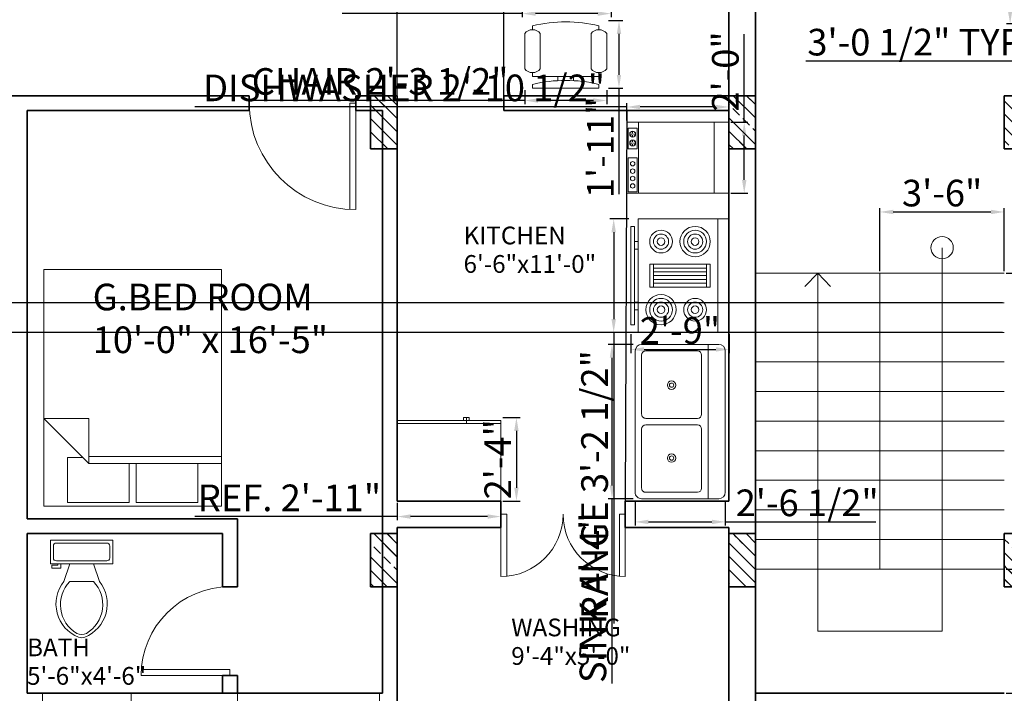
# Model space of a CAD drawing. Units: inches. Extents: x 2081 to 4786, y 1256 to 3802.
# Tile 3 of 7: x 2352 to 2685, y 1442 to 1670. Entities that reach past the tile are written whole.
import ezdxf

# ---------------------------------------------------------------- set-up
doc = ezdxf.new("R2010")
doc.units = ezdxf.units.IN
for name, color, linetype, lineweight in [('A-ANNO-DIMS', 18, 'Continuous', 18), ('A-AREA-IDEN', 18, 'Continuous', 18), ('A-COLS', 1, 'Continuous', 35), ('A-DOOR', 5, 'Continuous', 18), ('A-EQPM', 11, 'Continuous', 18), ('A-FLOR-CASE', 7, 'Continuous', 25), ('A-FLOR-FIXT', 18, 'Continuous', 18), ('A-FLOR-STRS', 7, 'Continuous', 18), ('A-FURN', 5, 'Continuous', 18), ('A-GLAZ', 11, 'Continuous', 18), ('A-WALL', 7, 'Continuous', 35)]:
    doc.layers.add(name, color=color, linetype=linetype, lineweight=lineweight)
doc.styles.get("Standard").update_dxf_attribs({"font": 'arial.ttf'})
doc.dimstyles.new('ISO-25', dxfattribs={"dimtxt": 9, "dimasz": 4.5, "dimexe": 1.25, "dimexo": 0.625, "dimtad": 1, "dimdec": 0, "dimlunit": 3, "dimtxsty": 'Standard', "dimcen": 2.5, "dimadec": 0, "dimazin": 0, "dimtfac": 1, "dimtdec": 0, "dimtmove": 0, "dimatfit": 3, "dimfxl": 1, "dimarcsym": 0})
pattern_1 = [(135, (1916.44, -3174.735), (-13.47038, -13.47038), []), (135, (1916.44, -3170.245), (-13.47038, -13.47038), []), (135, (1916.44, -3165.755), (-13.47038, -13.47038), []), (135, (1916.44, -3161.265), (-13.47038, -13.47038), [])]

# ---------------------------------------------------------------- blocks, each defined once
blk = doc.blocks.new('Bed - Queen')
for p, q in [((0, -80.00003), (0, 0)), ((0, 0), (59.99999, 0)), ((59.99999, 0), (59.99999, -80.00003)), ((7.99999, -1.2), (28.79998, -1.2)), ((7.99999, -14.4), (7.99999, -1.2)), ((28.79998, -1.2), (28.79998, -14.4)), ((31.19999, -1.2), (51.99999, -1.2)), ((31.19999, -14.4), (31.19999, -1.2)), ((51.99999, -1.2), (51.99999, -16.4)), ((0, -14.4), (44.8, -14.4)), ((59.99999, -29.6), (44.8, -14.4)), ((44.8, -14.4), (44.8, -29.6)), ((51.99999, -16.4), (46.79936, -16.4)), ((44.8, -16.8), (0, -16.8)), ((44.8, -29.6), (59.99999, -29.6)), ((59.99999, -80.00003), (0, -80.00003))]:
    blk.add_line(p, q)
blk = doc.blocks.new('Chair - Desk')
for p, q in [((-8.5, 0), (-8.5, -1)), ((-8.5, 0), (8.5, 0)), ((8.5, 0), (8.5, -1)), ((-2, -3), (-2, -1.9355)), ((2, -1.9576), (2, -3)), ((-10.5, -5), (-10.5, -14)), ((-8.5, -3), (-8.5, -4)), ((-8.5, -3), (8.5, -3)), ((-6.5, -14), (-6.5, -5)), ((6.5, -5), (6.5, -14)), ((8.5, -3), (8.5, -4)), ((10.5, -14), (10.5, -5)), ((-8.5, -15), (-8.5, -16)), ((8.5, -15), (8.5, -16))]:
    blk.add_line(p, q)
for centre, radius, start, end in [((0, 34.625), 36.625, 256.5803, 283.4197), ((-8.5, -6.5), 2.5, 36.8699, 143.1301), ((8.5, -6.5), 2.5, 36.8699, 143.1301), ((-8.5, -12.5), 2.5, 216.8699, 323.1301), ((8.5, -12.5), 2.5, 216.8699, 323.1301), ((0, 19.625), 36.625, 256.5803, 283.4197)]:
    blk.add_arc(centre, radius, start, end)
blk = doc.blocks.new('Range-Oven - 30 in top')
for p, q in [((0, -3), (30, -3)), ((12, -6), (18, -6)), ((13, -20), (13, -6)), ((14, -6), (14, -20)), ((15, -20), (15, -6)), ((16, -6), (16, -20)), ((17, -20), (17, -6)), ((18, -20), (12, -20)), ((6, -24), (6, -25)), ((8, -25), (8, -24)), ((22, -25), (22, -24)), ((24, -24), (24, -25))]:
    blk.add_line(p, q)
for points in [[(0, -24), (0, 0), (30, 0), (30, -24)], [(12, -21), (12, -5), (18, -5), (18, -21)], [(2, -26), (2, -25), (28, -25), (28, -26)]]:
    blk.add_lwpolyline(points, close=True)
for centre, radius in [((6, -9), 4), ((6, -9), 3), ((6, -9), 2), ((24, -9), 3), ((24, -9), 2), ((6, -9), 1), ((24, -9), 1), ((6, -18), 3), ((24, -18), 4), ((24, -18), 3), ((6, -18), 2), ((6, -18), 1), ((24, -18), 2), ((24, -18), 1)]:
    blk.add_circle(centre, radius)
blk = doc.blocks.new('Refrigerator-2 door - 36 in top')
for p, q in [((0, -26.999999), (36, -26.999999)), ((12, -26.999999), (12, -28.999999)), ((11, -27.999999), (11, -28.999999)), ((11, -28.999999), (13, -28.999999)), ((13, -28.999999), (13, -27.999999))]:
    blk.add_line(p, q)
blk.add_lwpolyline([(0, -27.999999), (0, 0), (36, 0), (36, -27.999999)], close=True)
blk = doc.blocks.new('Dishwasher')
for p, q in [((17, 32.75), (17, 33.5)), ((20, 32.75), (20, 33.5)), ((24, 30.5), (0, 30.5)), ((16, 32.5), (16.75, 32.5)), ((16.5, 32), (16.2942, 31.7942)), ((16.3156, 33.1843), (16.5, 33)), ((17, 32.25), (17, 31.5)), ((18, 32.5), (17.25, 32.5)), ((17.5, 33), (17.6938, 33.1938)), ((17.7061, 31.7939), (17.5, 32)), ((19, 32.5), (19.75, 32.5)), ((19.5, 32), (19.2942, 31.7942)), ((19.3156, 33.1843), (19.5, 33)), ((20, 32.25), (20, 31.5)), ((21, 32.5), (20.25, 32.5)), ((20.5, 33), (20.6938, 33.1938)), ((20.7061, 31.7939), (20.5, 32)), ((0, 5), (24, 5))]:
    blk.add_line(p, q)
for points in [[(0, 0), (0, 34.5), (24, 34.5), (24, 0)], [(0.5, 31), (0.5, 34), (12, 34), (12, 31)], [(15, 31), (15, 34), (22, 34), (22, 31)]]:
    blk.add_lwpolyline(points, close=True)
for centre, radius in [((17, 32.5), 1), ((20, 32.5), 1), ((2.5, 32.5), 0.75), ((5, 32.5), 0.75), ((7.5, 32.5), 0.75), ((10, 32.5), 0.75)]:
    blk.add_circle(centre, radius)
blk = doc.blocks.new('Sink-double - 36 in top')
for p, q in [((-18, -4), (18, -4)), ((-0.75, -18.5), (-0.75, -6.5)), ((0.75, -6.5), (0.75, -18.5))]:
    blk.add_line(p, q)
for points in [[(-16.5, 0), (16.5, 0)], [(-18, -19.5), (-18, -1.5)], [(18, -1.5), (18, -19.5)], [(-16.5, -18.5), (-16.5, -6.5)], [(-15.5, -5.5), (-1.75, -5.5)], [(1.75, -5.5), (15.5, -5.5)], [(16.5, -6.5), (16.5, -18.5)], [(-1.75, -19.5), (-15.5, -19.5)], [(15.5, -19.5), (1.75, -19.5)], [(16.5, -21), (-16.5, -21)]]:
    blk.add_lwpolyline(points)
for centre, radius in [((-8.5, -12.5), 1), ((-8.5, -12.5), 0.5), ((8.5, -12.5), 1), ((8.5, -12.5), 0.5)]:
    blk.add_circle(centre, radius)
for centre, radius, start, end in [((-16.5, -1.5), 1.5, 90, 180), ((16.5, -1.5), 1.5, 0, 90), ((-15.5, -6.5), 1, 90, 180), ((-1.75, -6.5), 1, 0, 90), ((1.75, -6.5), 1, 90, 180), ((15.5, -6.5), 1, 0, 90), ((-16.5, -19.5), 1.5, 180, 270), ((-15.5, -18.5), 1, 180, 270), ((-1.75, -18.5), 1, 270, 0), ((1.75, -18.5), 1, 180, 270), ((15.5, -18.5), 1, 270, 0), ((16.5, -19.5), 1.5, 270, 0)]:
    blk.add_arc(centre, radius, start, end)
blk = doc.blocks.new('Toilet - top')
for p, q in [((9.5, -6), (9.5, -2)), ((-10, -8.5), (-8, -8.5)), ((-10, -9.5), (-10, -8.5)), ((-7, -9.5), (-10, -9.5)), ((-8, -8.5), (-8, -8)), ((-7, -8), (-7, -9.5)), ((-4, -8), (-6, -14)), ((4, -8), (6, -14)), ((4, -14), (-4, -14))]:
    blk.add_line(p, q)
blk.add_lwpolyline([(10.5, -8), (10.5, 0), (-10.5, 0), (-10.5, -8)], close=True)
for points in [[(-9.5, -2), (-9.5, -6)], [(8.5, -1), (-8.5, -1)], [(-8.5, -7), (8.5, -7)]]:
    blk.add_lwpolyline(points)
for centre, radius, start, end in [((-8.62, -1.88), 0.884, 81.8699, 188.1301), ((8.62, -1.88), 0.884, 351.8699, 98.1301), ((-8.62, -6.12), 0.884, 171.8699, 278.1301), ((8.62, -6.12), 0.884, 261.8699, 8.1301), ((3.52, -21.58), 12.17, 141.4691, 247.9714), ((4.2, -21.82), 11.33, 136.3677, 238.9468), ((-3.52, -21.58), 12.17, 292.0284, 38.5307), ((-4.2, -21.82), 11.33, 301.053, 43.6321), ((0, -27.88), 4, 245.7318, 294.2682), ((0, -29), 4, 254.8605, 285.1395)]:
    blk.add_arc(centre, radius, start, end)
blk = doc.blocks.new('*D16')
at = {"layer": 'A-ANNO-DIMS', "color": 0, "lineweight": -2, "transparency": 16777216}
for p, q in [((2642.98, 1584.8), (2642.98, 1606.11)), ((2684.98, 1584.8), (2684.98, 1606.11)), ((2647.48, 1604.86), (2680.48, 1604.86))]:
    blk.add_line(p, q, dxfattribs=at)
at = {"layer": 'A-ANNO-DIMS', "color": 0, "transparency": 16777216}
for points in [[(2647.48, 1605.61), (2647.48, 1604.11), (2642.98, 1604.86)], [(2680.48, 1605.61), (2680.48, 1604.11), (2684.98, 1604.86)]]:
    blk.add_solid(points, dxfattribs=at)
at = {"layer": 'Defpoints', "color": 0, "transparency": 16777216}
for p in [(2684.98, 1604.86), (2642.98, 1584.17), (2684.98, 1584.17)]:
    blk.add_point(p, dxfattribs=at)
at = {"layer": 'A-ANNO-DIMS', "color": 0, "transparency": 16777216, "insert": (2663.98, 1610.08), "char_height": 9, "attachment_point": 5}
blk.add_mtext('3\'-6"', dxfattribs=at)
blk = doc.blocks.new('DOOR-PAIR-42IN')
for p, q in [((0, 42), (21, 42)), ((0, 40), (21, 40)), ((21, 42), (21, 40)), ((0, 2), (21, 2)), ((21, 0), (21, 2)), ((0, 0), (21, 0))]:
    blk.add_line(p, q)
for centre, start, end in [((21, 42), 180, 270), ((21, 0), 90, 180)]:
    blk.add_arc(centre, 21, start, end)
blk = doc.blocks.new('DOOR-SINGLE-36IN')
for p, q in [((34, 36), (34, 0)), ((36, 36), (36, 0)), ((36, 0), (34, 0))]:
    blk.add_line(p, q)
blk.add_arc((36, 0), 36, 90, 180)
blk = doc.blocks.new('DOOR-SINGLE-30IN')
for p, q in [((0, 30), (30, 30)), ((30, 30), (30, 28)), ((0, 28), (30, 28))]:
    blk.add_line(p, q)
blk.add_arc((30, 30), 30, 180, 270)
blk = doc.blocks.new('WINDOW-48IN')
for p, q in [((0, 0), (0, 9)), ((0, 9), (4, 9)), ((4, 9), (48, 9)), ((48, 0), (48, 9)), ((48, 6), (0, 6)), ((48, 4.5), (0, 4.5)), ((48, 3), (0, 3)), ((48, 0), (0, 0))]:
    blk.add_line(p, q)
blk = doc.blocks.new('WINDOW-30IN')
for p, q in [((0, 0), (0, 30)), ((0, 30), (9, 30)), ((3, 0), (3, 30)), ((4.5, 0), (4.5, 30)), ((6, 0), (6, 30)), ((9, 30), (9, 0)), ((9, 0), (0, 0))]:
    blk.add_line(p, q)
blk = doc.blocks.new('COLUMN-9X18IN')
h = blk.add_hatch()
h.set_pattern_fill('ANSI34', color=256, angle=90)
h.set_pattern_definition(pattern_1)
h.paths.add_polyline_path([(9, 18), (0, 18), (0, 0), (9, 0)])
h = blk.add_hatch()
h.set_pattern_fill('ANSI34', color=256, angle=90)
h.set_pattern_definition(pattern_1)
h.paths.add_polyline_path([(9, 18), (0, 18), (0, 0), (9, 0)])
h = blk.add_hatch()
h.set_pattern_fill('ANSI34', color=256, angle=90)
h.set_pattern_definition(pattern_1)
h.paths.add_polyline_path([(9, 18), (0, 18), (0, 0), (9, 0)])
h = blk.add_hatch()
h.set_pattern_fill('ANSI33', color=256, angle=90)
h.set_pattern_definition([(135, (1916.44, -3174.7355), (-4.490128, -4.490128), []), (135, (1916.44, -3170.2454), (-4.490128, -4.490128), [3.175, -1.5875])])
h.paths.add_polyline_path([(0, 0), (9, 0), (9, 18), (0, 18)])
for p, q in [((0, 0), (0, 18)), ((0, 18), (9, 18)), ((9, 18), (9, 0)), ((9, 0), (0, 0))]:
    blk.add_line(p, q)
blk = doc.blocks.new('*D53')
at = {"layer": 'A-ANNO-DIMS', "color": 0, "lineweight": -2, "transparency": 16777216}
for p, q in [((2523.02, 1646.06), (2523.02, 1641.28)), ((2550.71, 1646.06), (2550.71, 1641.28)), ((2523.02, 1642.53), (2429.87, 1642.53)), ((2546.21, 1642.53), (2527.52, 1642.53))]:
    blk.add_line(p, q, dxfattribs=at)
at = {"layer": 'A-ANNO-DIMS', "color": 0, "transparency": 16777216}
for points in [[(2527.52, 1643.28), (2527.52, 1641.78), (2523.02, 1642.53)], [(2546.21, 1643.28), (2546.21, 1641.78), (2550.71, 1642.53)]]:
    blk.add_solid(points, dxfattribs=at)
at = {"layer": 'Defpoints', "color": 0, "transparency": 16777216}
for p in [(2523.02, 1646.68), (2550.71, 1646.68), (2523.02, 1642.53)]:
    blk.add_point(p, dxfattribs=at)
at = {"layer": 'A-ANNO-DIMS', "color": 0, "transparency": 16777216, "insert": (2474.2, 1647.81), "char_height": 9, "attachment_point": 5}
blk.add_mtext('CHAIR 2\'-3 1/2"', dxfattribs=at)
blk = doc.blocks.new('*D54')
at = {"layer": 'A-ANNO-DIMS', "color": 0, "lineweight": -2, "transparency": 16777216}
for p, q in [((2551.33, 1669.53), (2556.11, 1669.53)), ((2554.86, 1665.03), (2554.86, 1651.18)), ((2551.33, 1646.68), (2556.11, 1646.68)), ((2554.86, 1646.68), (2554.86, 1610.86))]:
    blk.add_line(p, q, dxfattribs=at)
at = {"layer": 'A-ANNO-DIMS', "color": 0, "transparency": 16777216}
for points in [[(2554.11, 1665.03), (2555.61, 1665.03), (2554.86, 1669.53)], [(2554.11, 1651.18), (2555.61, 1651.18), (2554.86, 1646.68)]]:
    blk.add_solid(points, dxfattribs=at)
at = {"layer": 'Defpoints', "color": 0, "transparency": 16777216}
for p in [(2550.71, 1669.53), (2550.71, 1646.68), (2554.86, 1646.68)]:
    blk.add_point(p, dxfattribs=at)
at = {"layer": 'A-ANNO-DIMS', "color": 0, "transparency": 16777216, "insert": (2549.72, 1626.52), "char_height": 9, "attachment_point": 5, "rotation": 90}
blk.add_mtext('1\'-11"', dxfattribs=at)
blk = doc.blocks.new('*D55')
at = {"layer": 'A-ANNO-DIMS', "color": 0, "lineweight": -2, "transparency": 16777216}
for p, q in [((2686.95, 1752.41), (2686.95, 1850.7)), ((2698.93, 1752.41), (2685.7, 1752.41)), ((2686.95, 1672.91), (2686.95, 1747.91)), ((2698.93, 1668.41), (2685.7, 1668.41))]:
    blk.add_line(p, q, dxfattribs=at)
at = {"layer": 'A-ANNO-DIMS', "color": 0, "transparency": 16777216}
for points in [[(2686.2, 1747.91), (2687.7, 1747.91), (2686.95, 1752.41)], [(2686.2, 1672.91), (2687.7, 1672.91), (2686.95, 1668.41)]]:
    blk.add_solid(points, dxfattribs=at)
at = {"layer": 'Defpoints', "color": 0, "transparency": 16777216}
for p in [(2686.95, 1752.41), (2699.55, 1752.41), (2699.55, 1668.41)]:
    blk.add_point(p, dxfattribs=at)
at = {"layer": 'A-ANNO-DIMS', "color": 0, "transparency": 16777216, "insert": (2681.67, 1803.8), "char_height": 9, "attachment_point": 5, "rotation": 90}
blk.add_mtext('SOFA 7\'-0" TYP.', dxfattribs=at)
blk = doc.blocks.new('*D56')
at = {"layer": 'A-ANNO-DIMS', "color": 0, "lineweight": -2, "transparency": 16777216}
for p, q in [((2699.55, 1667.78), (2699.55, 1654.56)), ((2736.22, 1667.78), (2736.22, 1654.56)), ((2699.55, 1655.81), (2617.98, 1655.81)), ((2731.72, 1655.81), (2704.05, 1655.81))]:
    blk.add_line(p, q, dxfattribs=at)
at = {"layer": 'A-ANNO-DIMS', "color": 0, "transparency": 16777216}
for points in [[(2704.05, 1656.56), (2704.05, 1655.06), (2699.55, 1655.81)], [(2731.72, 1656.56), (2731.72, 1655.06), (2736.22, 1655.81)]]:
    blk.add_solid(points, dxfattribs=at)
at = {"layer": 'Defpoints', "color": 0, "transparency": 16777216}
for p in [(2699.55, 1668.41), (2736.22, 1668.41), (2699.55, 1655.81)]:
    blk.add_point(p, dxfattribs=at)
at = {"layer": 'A-ANNO-DIMS', "color": 0, "transparency": 16777216, "insert": (2656.52, 1661.09), "char_height": 9, "attachment_point": 5}
blk.add_mtext('3\'-0 1/2" TYP.', dxfattribs=at)
blk = doc.blocks.new('*D58')
at = {"layer": 'A-ANNO-DIMS', "color": 0, "lineweight": -2, "transparency": 16777216}
for p, q in [((2522.19, 1680.27), (2522.19, 1670.65)), ((2552.19, 1680.27), (2552.19, 1670.65)), ((2522.19, 1671.9), (2461.43, 1671.9)), ((2547.69, 1671.9), (2526.69, 1671.9))]:
    blk.add_line(p, q, dxfattribs=at)
at = {"layer": 'A-ANNO-DIMS', "color": 0, "transparency": 16777216}
for points in [[(2526.69, 1672.65), (2526.69, 1671.15), (2522.19, 1671.9)], [(2547.69, 1672.65), (2547.69, 1671.15), (2552.19, 1671.9)]]:
    blk.add_solid(points, dxfattribs=at)
at = {"layer": 'Defpoints', "color": 0, "transparency": 16777216}
for p in [(2522.19, 1680.9), (2552.19, 1680.9), (2522.19, 1671.9)]:
    blk.add_point(p, dxfattribs=at)
at = {"layer": 'A-ANNO-DIMS', "color": 0, "transparency": 16777216, "insert": (2489.56, 1677.12), "char_height": 9, "attachment_point": 5}
blk.add_mtext('2\'-6" TYP.', dxfattribs=at)
blk = doc.blocks.new('*D61')
at = {"layer": 'A-ANNO-DIMS', "color": 0, "lineweight": -2, "transparency": 16777216}
for p, q in [((2558.2, 1602.52), (2551.82, 1602.52)), ((2553.07, 1598.02), (2553.07, 1568.65)), ((2558.2, 1564.15), (2551.82, 1564.15)), ((2553.07, 1564.15), (2553.07, 1465.77))]:
    blk.add_line(p, q, dxfattribs=at)
at = {"layer": 'A-ANNO-DIMS', "color": 0, "transparency": 16777216}
for points in [[(2552.32, 1598.02), (2553.82, 1598.02), (2553.07, 1602.52)], [(2552.32, 1568.65), (2553.82, 1568.65), (2553.07, 1564.15)]]:
    blk.add_solid(points, dxfattribs=at)
at = {"layer": 'Defpoints', "color": 0, "transparency": 16777216}
for p in [(2558.83, 1602.52), (2553.07, 1564.15), (2558.83, 1564.15)]:
    blk.add_point(p, dxfattribs=at)
at = {"layer": 'A-ANNO-DIMS', "color": 0, "transparency": 16777216, "insert": (2547.79, 1512.71), "char_height": 9, "attachment_point": 5, "rotation": 90}
blk.add_mtext('RANGE 3\'-2 1/2"', dxfattribs=at)
blk = doc.blocks.new('*D62')
at = {"layer": 'A-ANNO-DIMS', "color": 0, "lineweight": -2, "transparency": 16777216}
for p, q in [((2558.83, 1563.53), (2558.83, 1557.15)), ((2592.08, 1563.53), (2592.08, 1557.15)), ((2563.33, 1558.4), (2587.58, 1558.4))]:
    blk.add_line(p, q, dxfattribs=at)
at = {"layer": 'A-ANNO-DIMS', "color": 0, "transparency": 16777216}
for points in [[(2563.33, 1559.15), (2563.33, 1557.65), (2558.83, 1558.4)], [(2587.58, 1559.15), (2587.58, 1557.65), (2592.08, 1558.4)]]:
    blk.add_solid(points, dxfattribs=at)
at = {"layer": 'Defpoints', "color": 0, "transparency": 16777216}
for p in [(2558.83, 1564.15), (2592.08, 1564.15), (2592.08, 1558.4)]:
    blk.add_point(p, dxfattribs=at)
at = {"layer": 'A-ANNO-DIMS', "color": 0, "transparency": 16777216, "insert": (2575.45, 1563.62), "char_height": 9, "attachment_point": 5}
blk.add_mtext('2\'-9"', dxfattribs=at)
blk = doc.blocks.new('*D65')
at = {"layer": 'A-ANNO-DIMS', "color": 0, "lineweight": -2, "transparency": 16777216}
for p, q in [((2557.48, 1640.35), (2411.58, 1640.35)), ((2557.48, 1635.8), (2557.48, 1641.6)), ((2587.48, 1640.35), (2561.98, 1640.35)), ((2591.98, 1635.8), (2591.98, 1641.6))]:
    blk.add_line(p, q, dxfattribs=at)
at = {"layer": 'A-ANNO-DIMS', "color": 0, "transparency": 16777216}
for points in [[(2561.98, 1641.1), (2561.98, 1639.6), (2557.48, 1640.35)], [(2587.48, 1641.1), (2587.48, 1639.6), (2591.98, 1640.35)]]:
    blk.add_solid(points, dxfattribs=at)
at = {"layer": 'Defpoints', "color": 0, "transparency": 16777216}
for p in [(2557.48, 1640.35), (2557.48, 1635.17), (2591.98, 1635.17)]:
    blk.add_point(p, dxfattribs=at)
at = {"layer": 'A-ANNO-DIMS', "color": 0, "transparency": 16777216, "insert": (2482.28, 1645.63), "char_height": 9, "attachment_point": 5}
blk.add_mtext('DISHWASHER 2\'-10 1/2"', dxfattribs=at)
blk = doc.blocks.new('*D66')
at = {"layer": 'A-ANNO-DIMS', "color": 0, "lineweight": -2, "transparency": 16777216}
for p, q in [((2597.16, 1635.17), (2597.16, 1665)), ((2592.61, 1635.17), (2598.41, 1635.17)), ((2597.16, 1615.67), (2597.16, 1630.67)), ((2592.61, 1611.17), (2598.41, 1611.17))]:
    blk.add_line(p, q, dxfattribs=at)
at = {"layer": 'A-ANNO-DIMS', "color": 0, "transparency": 16777216}
for points in [[(2596.41, 1630.67), (2597.91, 1630.67), (2597.16, 1635.17)], [(2596.41, 1615.67), (2597.91, 1615.67), (2597.16, 1611.17)]]:
    blk.add_solid(points, dxfattribs=at)
at = {"layer": 'Defpoints', "color": 0, "transparency": 16777216}
for p in [(2591.98, 1635.17), (2597.16, 1635.17), (2591.98, 1611.17)]:
    blk.add_point(p, dxfattribs=at)
at = {"layer": 'A-ANNO-DIMS', "color": 0, "transparency": 16777216, "insert": (2591.94, 1652.34), "char_height": 9, "attachment_point": 5, "rotation": 90}
blk.add_mtext('2\'-0"', dxfattribs=at)
blk = doc.blocks.new('*D69')
at = {"layer": 'A-ANNO-DIMS', "color": 0, "lineweight": -2, "transparency": 16777216}
for p, q in [((2559.7, 1560.09), (2551.25, 1560.09)), ((2552.5, 1555.59), (2552.5, 1512.44)), ((2559.7, 1507.94), (2551.25, 1507.94)), ((2552.5, 1507.94), (2552.5, 1445.47))]:
    blk.add_line(p, q, dxfattribs=at)
at = {"layer": 'A-ANNO-DIMS', "color": 0, "transparency": 16777216}
for points in [[(2551.75, 1555.59), (2553.25, 1555.59), (2552.5, 1560.09)], [(2551.75, 1512.44), (2553.25, 1512.44), (2552.5, 1507.94)]]:
    blk.add_solid(points, dxfattribs=at)
at = {"layer": 'Defpoints', "color": 0, "transparency": 16777216}
for p in [(2560.32, 1560.09), (2552.5, 1507.94), (2560.32, 1507.94)]:
    blk.add_point(p, dxfattribs=at)
at = {"layer": 'A-ANNO-DIMS', "color": 0, "transparency": 16777216, "insert": (2547.22, 1474.45), "char_height": 9, "attachment_point": 5, "rotation": 90}
blk.add_mtext('SINK 4\'-4"', dxfattribs=at)
blk = doc.blocks.new('*D70')
at = {"layer": 'A-ANNO-DIMS', "color": 0, "lineweight": -2, "transparency": 16777216}
for p, q in [((2560.32, 1507.31), (2560.32, 1498.86)), ((2590.75, 1507.31), (2590.75, 1498.86)), ((2564.82, 1500.11), (2586.25, 1500.11)), ((2590.75, 1500.11), (2641.55, 1500.11))]:
    blk.add_line(p, q, dxfattribs=at)
at = {"layer": 'A-ANNO-DIMS', "color": 0, "transparency": 16777216}
for points in [[(2564.82, 1500.86), (2564.82, 1499.36), (2560.32, 1500.11)], [(2586.25, 1500.86), (2586.25, 1499.36), (2590.75, 1500.11)]]:
    blk.add_solid(points, dxfattribs=at)
at = {"layer": 'Defpoints', "color": 0, "transparency": 16777216}
for p in [(2560.32, 1507.94), (2590.75, 1507.94), (2590.75, 1500.11)]:
    blk.add_point(p, dxfattribs=at)
at = {"layer": 'A-ANNO-DIMS', "color": 0, "transparency": 16777216, "insert": (2618.4, 1505.39), "char_height": 9, "attachment_point": 5}
blk.add_mtext('2\'-6 1/2"', dxfattribs=at)
blk = doc.blocks.new('*D75')
at = {"layer": 'A-ANNO-DIMS', "color": 0, "lineweight": -2, "transparency": 16777216}
for p, q in [((2479.98, 1506.55), (2479.98, 1500.67)), ((2514.98, 1506.55), (2514.98, 1500.67)), ((2479.98, 1501.92), (2411.65, 1501.92)), ((2510.48, 1501.92), (2484.48, 1501.92))]:
    blk.add_line(p, q, dxfattribs=at)
at = {"layer": 'A-ANNO-DIMS', "color": 0, "transparency": 16777216}
for points in [[(2484.48, 1502.67), (2484.48, 1501.17), (2479.98, 1501.92)], [(2510.48, 1502.67), (2510.48, 1501.17), (2514.98, 1501.92)]]:
    blk.add_solid(points, dxfattribs=at)
at = {"layer": 'Defpoints', "color": 0, "transparency": 16777216}
for p in [(2479.98, 1507.17), (2514.98, 1507.17), (2479.98, 1501.92)]:
    blk.add_point(p, dxfattribs=at)
at = {"layer": 'A-ANNO-DIMS', "color": 0, "transparency": 16777216, "insert": (2443.57, 1507.07), "char_height": 9, "attachment_point": 5}
blk.add_mtext('REF. 2\'-11"', dxfattribs=at)
blk = doc.blocks.new('*D76')
at = {"layer": 'A-ANNO-DIMS', "color": 0, "lineweight": -2, "transparency": 16777216}
for p, q in [((2515.61, 1535.37), (2521.48, 1535.37)), ((2520.23, 1530.87), (2520.23, 1511.67)), ((2515.61, 1507.17), (2521.48, 1507.17))]:
    blk.add_line(p, q, dxfattribs=at)
at = {"layer": 'A-ANNO-DIMS', "color": 0, "transparency": 16777216}
for points in [[(2519.48, 1530.87), (2520.98, 1530.87), (2520.23, 1535.37)], [(2519.48, 1511.67), (2520.98, 1511.67), (2520.23, 1507.17)]]:
    blk.add_solid(points, dxfattribs=at)
at = {"layer": 'Defpoints', "color": 0, "transparency": 16777216}
for p in [(2514.98, 1535.37), (2514.98, 1507.17), (2520.23, 1507.17)]:
    blk.add_point(p, dxfattribs=at)
at = {"layer": 'A-ANNO-DIMS', "color": 0, "transparency": 16777216, "insert": (2515.09, 1521.27), "char_height": 9, "attachment_point": 5, "rotation": 90}
blk.add_mtext('2\'-4"', dxfattribs=at)
blk = doc.blocks.new('*D78')
at = {"layer": 'A-ANNO-DIMS', "color": 0, "lineweight": -2, "transparency": 16777216}
for p, q in [((2479.98, 1626.8), (2479.98, 2072.92)), ((2484.48, 2071.67), (2511.48, 2071.67)), ((2515.98, 1639.8), (2515.98, 2072.92))]:
    blk.add_line(p, q, dxfattribs=at)
at = {"layer": 'A-ANNO-DIMS', "color": 0, "transparency": 16777216}
for points in [[(2484.48, 2072.42), (2484.48, 2070.92), (2479.98, 2071.67)], [(2511.48, 2072.42), (2511.48, 2070.92), (2515.98, 2071.67)]]:
    blk.add_solid(points, dxfattribs=at)
at = {"layer": 'Defpoints', "color": 0, "transparency": 16777216}
for p in [(2515.98, 2071.67), (2515.98, 1639.17), (2479.98, 1626.17)]:
    blk.add_point(p, dxfattribs=at)
at = {"layer": 'A-ANNO-DIMS', "color": 0, "transparency": 16777216, "insert": (2497.98, 2076.9), "char_height": 9, "attachment_point": 5}
blk.add_mtext('3\'-0"', dxfattribs=at)
blk = doc.blocks.new('*D79')
at = {"layer": 'A-ANNO-DIMS', "color": 0, "lineweight": -2, "transparency": 16777216}
for p, q in [((2685.61, 1584.17), (3154.73, 1584.17)), ((3153.48, 1488.67), (3153.48, 1579.67)), ((2685.61, 1484.17), (3154.73, 1484.17))]:
    blk.add_line(p, q, dxfattribs=at)
at = {"layer": 'A-ANNO-DIMS', "color": 0, "transparency": 16777216}
for points in [[(3152.73, 1579.67), (3154.23, 1579.67), (3153.48, 1584.17)], [(3152.73, 1488.67), (3154.23, 1488.67), (3153.48, 1484.17)]]:
    blk.add_solid(points, dxfattribs=at)
at = {"layer": 'Defpoints', "color": 0, "transparency": 16777216}
for p in [(2684.98, 1584.17), (3153.48, 1584.17), (2684.98, 1484.17)]:
    blk.add_point(p, dxfattribs=at)
at = {"layer": 'A-ANNO-DIMS', "color": 0, "transparency": 16777216, "insert": (3148.26, 1534.17), "char_height": 9, "attachment_point": 5, "rotation": 90}
blk.add_mtext('8\'-4"', dxfattribs=at)
blk = doc.blocks.new('*D80')
at = {"layer": 'A-ANNO-DIMS', "color": 0, "lineweight": -2, "transparency": 16777216}
for p, q in [((2685.61, 1484.17), (3154.73, 1484.17)), ((3153.48, 1446.67), (3153.48, 1479.67)), ((2685.61, 1442.17), (3154.73, 1442.17))]:
    blk.add_line(p, q, dxfattribs=at)
at = {"layer": 'A-ANNO-DIMS', "color": 0, "transparency": 16777216}
for points in [[(3152.73, 1479.67), (3154.23, 1479.67), (3153.48, 1484.17)], [(3152.73, 1446.67), (3154.23, 1446.67), (3153.48, 1442.17)]]:
    blk.add_solid(points, dxfattribs=at)
at = {"layer": 'Defpoints', "color": 0, "transparency": 16777216}
for p in [(2684.98, 1484.17), (3153.48, 1484.17), (2684.98, 1442.17)]:
    blk.add_point(p, dxfattribs=at)
at = {"layer": 'A-ANNO-DIMS', "color": 0, "transparency": 16777216, "insert": (3148.26, 1463.17), "char_height": 9, "attachment_point": 5, "rotation": 90}
blk.add_mtext('3\'-6"', dxfattribs=at)
blk = doc.blocks.new('*D81')
at = {"layer": 'A-ANNO-DIMS', "color": 0, "lineweight": -2, "transparency": 16777216}
for p, q in [((2154.48, 1578.67), (2154.48, 1615.34)), ((2684.36, 1574.17), (2153.23, 1574.17)), ((2154.48, 1564.17), (2154.48, 1574.17)), ((2684.36, 1564.17), (2153.23, 1564.17)), ((2154.48, 1559.67), (2154.48, 1555.17))]:
    blk.add_line(p, q, dxfattribs=at)
at = {"layer": 'A-ANNO-DIMS', "color": 0, "transparency": 16777216}
for points in [[(2153.73, 1578.67), (2155.23, 1578.67), (2154.48, 1574.17)], [(2153.73, 1559.67), (2155.23, 1559.67), (2154.48, 1564.17)]]:
    blk.add_solid(points, dxfattribs=at)
at = {"layer": 'Defpoints', "color": 0, "transparency": 16777216}
for p in [(2154.48, 1574.17), (2684.98, 1574.17), (2684.98, 1564.17)]:
    blk.add_point(p, dxfattribs=at)
at = {"layer": 'A-ANNO-DIMS', "color": 0, "transparency": 16777216, "insert": (2149.26, 1599.26), "char_height": 9, "attachment_point": 5, "rotation": 90}
blk.add_mtext('0\'-10"', dxfattribs=at)

msp = doc.modelspace()

# ---------------------------------------------------------------- linework, layer by layer
at = {"layer": 'A-FLOR-CASE'}
msp.add_line((2557.48, 1639.17), (2556.98, 1507.17), dxfattribs=at)
at = {"layer": 'A-FLOR-STRS'}
for p, q in [((2663.98, 1584.17), (2663.98, 1592.79)), ((2684.98, 1584.17), (2600.98, 1584.17)), ((2621.98, 1584.17), (2617.64, 1579.7)), ((2621.98, 1463.17), (2621.98, 1584.17)), ((2621.98, 1584.17), (2626.33, 1579.7)), ((2642.98, 1484.17), (2642.98, 1584.17)), ((2663.98, 1484.17), (2663.98, 1584.17)), ((2684.98, 1574.17), (2600.98, 1574.17)), ((2684.98, 1564.17), (2600.98, 1564.17)), ((2684.98, 1554.17), (2600.98, 1554.17)), ((2684.98, 1544.17), (2600.98, 1544.17)), ((2684.98, 1534.17), (2600.98, 1534.17)), ((2684.98, 1524.17), (2600.98, 1524.17)), ((2684.98, 1514.17), (2600.98, 1514.17)), ((2684.98, 1504.17), (2600.98, 1504.17)), ((2684.98, 1494.17), (2600.98, 1494.17)), ((2684.98, 1484.17), (2600.98, 1484.17)), ((2663.98, 1484.17), (2663.98, 1463.17)), ((2663.98, 1463.17), (2621.98, 1463.17))]:
    msp.add_line(p, q, dxfattribs=at)
msp.add_circle((2663.98, 1592.79), 3.76, dxfattribs=at)
at = {"layer": 'A-WALL'}
for p, q in [((2591.98, 1644.17), (2591.98, 1780.17)), ((2600.98, 1433.17), (2600.98, 1780.17)), ((2343.98, 1644.17), (2429.98, 1644.17)), ((2429.98, 1639.17), (2429.98, 1644.17)), ((2465.98, 1639.17), (2465.98, 1644.17)), ((2465.98, 1644.17), (2479.98, 1644.17)), ((2479.98, 1507.17), (2479.98, 1644.17)), ((2515.98, 1639.17), (2515.98, 1644.17)), ((2515.98, 1644.17), (2591.98, 1644.17)), ((2354.98, 1639.17), (2429.98, 1639.17)), ((2354.98, 1501.17), (2354.98, 1639.17)), ((2465.98, 1639.17), (2474.98, 1639.17)), ((2474.98, 1442.17), (2474.98, 1639.17)), ((2515.98, 1639.17), (2591.98, 1639.17)), ((2591.98, 1507.17), (2591.98, 1639.17)), ((2514.98, 1507.17), (2479.98, 1507.17)), ((2514.98, 1507.17), (2514.98, 1498.17)), ((2591.98, 1507.17), (2556.98, 1507.17)), ((2556.98, 1507.17), (2556.98, 1498.17)), ((2425.98, 1501.17), (2354.98, 1501.17)), ((2425.98, 1478.17), (2425.98, 1501.17)), ((2479.98, 1438.17), (2479.98, 1498.17)), ((2514.98, 1498.17), (2479.98, 1498.17)), ((2591.98, 1498.17), (2556.98, 1498.17)), ((2591.98, 1438.17), (2591.98, 1498.17)), ((2354.98, 1442.17), (2354.98, 1496.17)), ((2420.98, 1496.17), (2354.98, 1496.17)), ((2420.98, 1478.17), (2420.98, 1496.17)), ((2474.98, 1496.17), (2470.98, 1496.17)), ((2425.98, 1478.17), (2420.98, 1478.17)), ((2474.98, 1478.17), (2470.98, 1478.17)), ((2420.98, 1442.17), (2420.98, 1448.17)), ((2425.98, 1448.17), (2420.98, 1448.17)), ((2425.98, 1442.17), (2425.98, 1448.17)), ((2474.98, 1442.17), (2354.98, 1442.17)), ((2684.98, 1442.17), (2600.98, 1442.17))]:
    msp.add_line(p, q, dxfattribs=at)

# ---------------------------------------------------------------- block references
at = {"layer": 'A-COLS'}
for p in [(2470.98, 1626.17), (2591.98, 1626.17), (2684.98, 1626.17), (2470.98, 1478.17), (2591.98, 1478.17), (2684.98, 1478.17)]:
    msp.add_blockref('COLUMN-9X18IN', p, dxfattribs=at)
at = {"layer": 'A-DOOR', "extrusion": (0, 0, -1), "zscale": -1, "rotation": 180}
for name, p in [('DOOR-SINGLE-36IN', (-2429.98, 1641.67)), ('DOOR-SINGLE-30IN', (-2393.48, 1478.17))]:
    msp.add_blockref(name, p, dxfattribs=at)
at = {"layer": 'A-DOOR', "rotation": 89.99999999999969}
msp.add_blockref('DOOR-PAIR-42IN', (2556.98, 1481.67), dxfattribs=at)
at = {"layer": 'A-EQPM', "rotation": 90}
msp.add_blockref('Dishwasher', (2591.98, 1611.17), dxfattribs=at)
at = {"layer": 'A-EQPM'}
for name, p, xscale, yscale, zscale, rotation in [('Range-Oven - 30 in top', (2592.08, 1602.52), 1.278805072528203, 1.278805072528203, 1.278805072528203, 270), ('Refrigerator-2 door - 36 in top', (2514.98, 1507.17), 0.9722222222222221, 0.9722222222222221, 0.9722222222222221, 180)]:
    msp.add_blockref(name, p, dxfattribs=dict(at, xscale=xscale, yscale=yscale, zscale=zscale, rotation=rotation))
at = {"layer": 'A-FLOR-FIXT', "xscale": 1.448797080044571, "yscale": 1.448797080044571, "zscale": 1.448797080044571, "rotation": 270}
msp.add_blockref('Sink-double - 36 in top', (2590.75, 1534.01), dxfattribs=at)
at = {"layer": 'A-FLOR-FIXT'}
msp.add_blockref('Toilet - top', (2373.39, 1493.97), dxfattribs=at)
at = {"layer": 'A-FURN', "xscale": 1.318343889107896, "yscale": 1.318343889107896, "zscale": 1.318343889107896, "rotation": 180}
msp.add_blockref('Chair - Desk', (2536.87, 1646.68), dxfattribs=at)
at = {"layer": 'A-FURN', "rotation": 180}
msp.add_blockref('Bed - Queen', (2420.61, 1505.46), dxfattribs=at)
at = {"layer": 'A-GLAZ', "rotation": 270.0000000000024}
msp.add_blockref('WINDOW-30IN', (2360.18, 1442.17), dxfattribs=at)
at = {"layer": 'A-GLAZ'}
msp.add_blockref('WINDOW-48IN', (2426.04, 1433.17), dxfattribs=at)

# ---------------------------------------------------------------- texts
at = {"layer": 'A-AREA-IDEN'}
for s, height, p in [('KITCHEN', 6, (2502.37, 1593.92)), ('6\'-6"x11\'-0"', 6, (2502.37, 1584.29)), ('G.BED ROOM', 9, (2377.12, 1571.62)), ('10\'-0" x 16\'-5"', 9, (2377.12, 1557.16)), ('WASHING', 6, (2518.48, 1461.44)), ('BATH', 6, (2354.98, 1454.7)), ('9\'-4"x5\'-0"', 6, (2518.48, 1451.8)), ('5\'-6"x4\'-6"', 6, (2354.98, 1445.06))]:
    msp.add_text(s, height=height, dxfattribs=at).set_placement(p)

# ---------------------------------------------------------------- dimensions: what is measured, and where the dimension line sits
at = {"layer": 'A-ANNO-DIMS'}
for base, p1, p2, override, picture, middle in [((2515.98, 2071.67), (2479.98, 1626.17), (2515.98, 1639.17), {"dimdec": 1, "dimlfac": 1, "dimrnd": 0, "dimzin": 1, "dimdsep": 46, "dimlunit": 4, "dimfrac": 2}, '*D78', (2497.98, 2076.9)), ((2684.98, 1604.86), (2642.98, 1584.17), (2684.98, 1584.17), {"dimclrd": 0, "dimclre": 0, "dimclrt": 0}, '*D16', (2663.98, 1610.08)), ((2592.0762, 1558.3968), (2558.8273, 1564.1514), (2592.0762, 1564.1514), {"dimdec": 1, "dimlfac": 1, "dimrnd": 0, "dimzin": 1, "dimdsep": 46, "dimlunit": 4, "dimfrac": 2}, '*D62', (2575.4517, 1563.6169)), ((2590.75, 1500.11), (2560.32, 1507.94), (2590.75, 1507.94), {"dimdec": 1, "dimlfac": 1, "dimrnd": 0, "dimzin": 1, "dimdsep": 46, "dimlunit": 4, "dimfrac": 2}, '*D70', (2618.4, 1505.39))]:
    dim = msp.add_linear_dim(base=base, p1=p1, p2=p2, dimstyle='ISO-25', override=override, dxfattribs=at)
    dim.commit()
    dim.dimension.update_dxf_attribs({"geometry": picture, "text_midpoint": middle})
for base, p1, p2, angle, text, picture, middle in [((2686.95, 1752.41), (2699.55, 1668.41), (2699.55, 1752.41), 90, 'SOFA <> TYP.', '*D55', (2681.67, 1803.8)), ((2522.19, 1671.9), (2552.19, 1680.9), (2522.19, 1680.9), 180, '<> TYP.', '*D58', (2489.56, 1677.12)), ((2699.55, 1655.81), (2736.22, 1668.41), (2699.55, 1668.41), 180, '<> TYP.', '*D56', (2656.52, 1661.09)), ((2557.48, 1640.35), (2591.98, 1635.17), (2557.48, 1635.17), 180, 'DISHWASHER <>', '*D65', (2482.28, 1645.63)), ((2523.02, 1642.53), (2550.71, 1646.68), (2523.02, 1646.68), 180, 'CHAIR <>', '*D53', (2474.2, 1647.81)), ((2553.07, 1564.15), (2558.83, 1602.52), (2558.83, 1564.15), 270, 'RANGE <>', '*D61', (2547.79, 1512.71)), ((2552.4981, 1507.9357), (2560.3216, 1560.0924), (2560.3216, 1507.9357), 270, 'SINK <>', '*D69', (2547.2196, 1474.4509)), ((2479.98, 1501.92), (2514.98, 1507.17), (2479.98, 1507.17), 180, 'REF. <>', '*D75', (2443.57, 1507.07))]:
    dim = msp.add_linear_dim(base=base, p1=p1, p2=p2, angle=angle, text=text, dimstyle='ISO-25', override={"dimdec": 1, "dimlfac": 1, "dimrnd": 0, "dimzin": 1, "dimdsep": 46, "dimlunit": 4, "dimfrac": 2}, dxfattribs=at)
    dim.commit()
    dim.dimension.update_dxf_attribs({"geometry": picture, "text_midpoint": middle})
for base, p1, p2, angle, picture, middle in [((2554.8618, 1646.6831), (2550.709, 1669.5344), (2550.709, 1646.6831), 270, '*D54', (2549.7184, 1626.5233)), ((2597.16, 1635.17), (2591.98, 1611.17), (2591.98, 1635.17), 90, '*D66', (2591.94, 1652.34)), ((2154.48, 1574.17), (2684.98, 1564.17), (2684.98, 1574.17), 90, '*D81', (2149.26, 1599.26)), ((3153.48, 1584.17), (2684.98, 1484.17), (2684.98, 1584.17), 90, '*D79', (3148.26, 1534.17)), ((2520.23, 1507.17), (2514.98, 1535.37), (2514.98, 1507.17), 270, '*D76', (2515.09, 1521.27)), ((3153.48, 1484.17), (2684.98, 1442.17), (2684.98, 1484.17), 90, '*D80', (3148.26, 1463.17))]:
    dim = msp.add_linear_dim(base=base, p1=p1, p2=p2, angle=angle, dimstyle='ISO-25', override={"dimdec": 1, "dimlfac": 1, "dimrnd": 0, "dimzin": 1, "dimdsep": 46, "dimlunit": 4, "dimfrac": 2}, dxfattribs=at)
    dim.commit()
    dim.dimension.update_dxf_attribs({"geometry": picture, "text_midpoint": middle})

doc.saveas('drawing.dxf')
